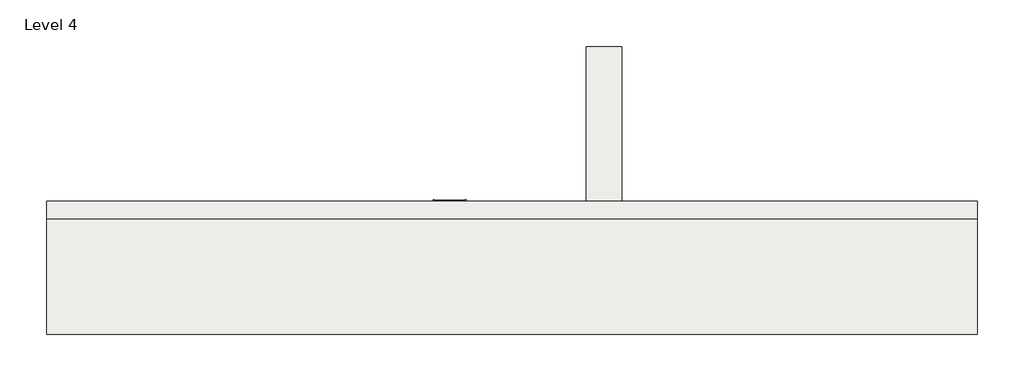
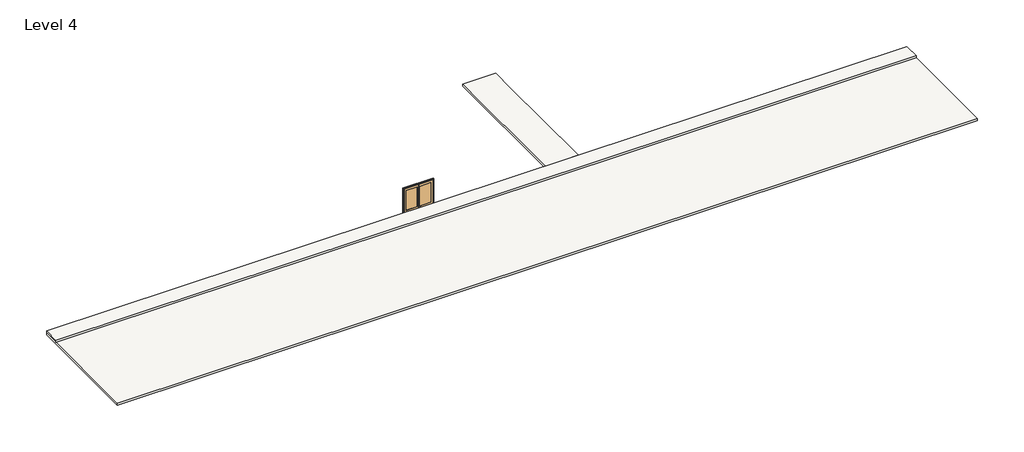
# One storey: 3 slabs, 1 door.
"""IFC4 building model written with IfcOpenShell, lengths in millimetres."""

from ifc_helpers import new_model, si_unit, frame, origin, place, context, project, spatial, polyline, outline, extrude, faceted_brep, transform, mapped, element, save
from components import garage_timber_side_hung_1_2271_x_2052mm_efc604d9

model = new_model("IFC4")

# Units and contexts
model_context = context("Model", 3, world=origin())
ifc_project = project(units=[si_unit("LENGTHUNIT", "METRE", prefix="MILLI")], contexts=[model_context])

# Site, building, storey
site = spatial("IfcSite", under=ifc_project)
building = spatial("IfcBuilding", under=site)
storey = spatial("IfcBuildingStorey", under=building, Name="Level 4", Elevation=-609.6)

# Door
placement = place(None, origin())
garage_timber_side_hung_1_2271_x_2052mm_shape = garage_timber_side_hung_1_2271_x_2052mm_efc604d9(model_context)
element("IfcDoor", 1, ObjectType="Garage - Timber Side Hung (1) : 2271 x 2052mm", at=placement, inside=storey, context=model_context, shape_type="MappedRepresentation", body=[
    mapped(garage_timber_side_hung_1_2271_x_2052mm_shape, transform((-4812.7201068, -6927.4122986, -609.6), x_axis=(-1.0, 0.0, 0.0), y_axis=(0.0, -1.0, 0.0), z_axis=(0.0, 0.0, 1.0))),
])

# Slabs
element("IfcSlab", 2, ObjectType="2' 3", at=placement, inside=storey, context=model_context, shape_type="SweptSolid", body=[
    extrude(outline(polyline([(31509.2798932, -7054.4122986), (31509.2798932, -16198.4122986), (-32536.8201068, -16198.4122986), (-32536.8201068, -7054.4122986), (31509.2798932, -7054.4122986)])), frame((0.0, 0.0, -762.0), z_axis=(0.0, 0.0, 1.0), x_axis=(1.0, 0.0, 0.0)), (0.0, 0.0, 1.0), 152.4),
])
element("IfcSlab", 3, ObjectType="2' 4", at=placement, inside=storey, context=model_context, shape_type="SweptSolid", body=[
    extrude(outline(polyline([(31509.2798932, -7054.4122986), (31509.2798932, -8273.6122986), (-32536.8201068, -8273.6122986), (-32536.8201068, -7054.4122986), (31509.2798932, -7054.4122986)])), frame((0.0, 0.0, -609.6), z_axis=(0.0, 0.0, 1.0), x_axis=(1.0, 0.0, 0.0)), (0.0, 0.0, 1.0), 152.4),
])
element("IfcSlab", 4, ObjectType="6\"", at=placement, inside=storey, context=model_context, shape_type="Brep", body=[
    faceted_brep([(7049.0798932, 3588.1877014, -609.6), (7049.0798932, -7054.4122986, -609.6), (4597.9798932, -7054.4122986, -609.6), (4597.9798932, 3588.1877014, -609.6), (7049.0798932, 3588.1877014, -457.2), (4597.9798932, 3588.1877014, -457.2), (4597.9798932, -7054.4122986, -457.2), (7049.0798932, -7054.4122986, -457.2), (7049.0798932, -6800.4122986, -457.2), (7049.0798932, 1746.6877014, -457.2)], [[[0, 1, 2, 3]], [[4, 5, 6, 7, 8, 9]], [[1, 0, 4, 9, 8, 7]], [[2, 1, 7, 6]], [[3, 2, 6, 5]], [[0, 3, 5, 4]]]),
])

save(model, "model.ifc")

# Revit data of these elements
# Type "Garage - Timber Side Hung (1) : 2271 x 2052mm"
#   Type Mark = "13"
#   Type Comments = "External Garage"
#   Operation = "DoubleDoorSingleSwing"
#   Manufacturer = "Revit"
#   Keynote = "L20"
#   Wrap Layers (Ext) from Ext = 0' - 4.03543"
#   Wrap Layers (Int) from Ext = 0' - 6.98819"
#   Thickness = 0' - 1.25984"
#   Stile Top Rail = 0' - 7.87402"
#   Stile Shutting = 0' - 3.93701"
#   Stile Lock Rail = 0' - 7.87402"
#   Stile Hanging = 0' - 6.88976"
#   Stile Bottom Rail = 0' - 9.84252"
#   Rough Width = 7' - 5.40945"
#   Rough Height = 6' - 8.7874"
#   O/A Frame Width = 0' - 2.51969"
#   Handle Z Distance = 3' - 5.33858"
#   Glazing Panel Height = 1' - 5.71654"
#   FrameWidth = 0' - 1.65354"
#   FrameOffset - External = 0' - 0.98425"
#   FrameDepth = 0' - 3.50394"
#   Door Panel Thickness = 0' - 1.25984"
#   Height = 6' - 8.7874"
#   Structural Tolerance = 0' - 0.31496"
#   Tolerance = 0' - 0.11811"
#   Undercut = 0' - 0.3937"
#   Width = 7' - 5.40945"
#   Cavity Closer Width = 0' - 1.9685"
#   Cavity Closer Offset from Ext = 0' - 4.03543"
#   Cavity Closer Depth = 0' - 2.95276"
#   Vis - Cavity Closers = yes
#   Function = 1
#   Material Door = Door - Panel
#   Wall Closure = (empty or 0)
# Type "2' 3"
#   Assembly Code = "B1010"
#   Function = 0
#   Layers, outside or top first: 0' - 6" "road" (function 1)
# Type "2' 4"
#   Assembly Code = "B1010"
#   Function = 0
#   Layers, outside or top first: 0' - 6" "road(1)" (function 1)
# Type "6\""
#   Assembly Code = "B1010"
#   Function = 0
#   Layers, outside or top first: 0' - 6" "0 floor outer" (function 1)
# Element 1 (IfcDoor, "Garage - Timber Side Hung (1) : 2271 x 2052mm")
#   Phase Created = New Construction
#   Materials on its faces: "Door - Panel"
# Element 2 (IfcSlab, "2' 3")
#   Height Offset From Level = 0' - 0"
#   Phase Created = New Construction
#   Materials on its faces: "road"
# Element 3 (IfcSlab, "2' 4")
#   Height Offset From Level = 0' - 6"
#   Phase Created = New Construction
#   Materials on its faces: "road(1)"
# Element 4 (IfcSlab, "6\"")
#   Height Offset From Level = 0' - 6"
#   Phase Created = New Construction
#   Materials on its faces: "0 floor outer", "0 olive green light"
# Materials
#   "Door - Panel": class "Wood", colour RGB 210 159 95, transparency 0, Cost = 0
#   "road": class "Generic", colour RGB 120 120 120, transparency 0, Cost = 0
#   "road(1)": class "Generic", colour RGB 120 120 120, transparency 0, Cost = 0
#   "0 floor outer": class "Generic", colour RGB 120 120 120, transparency 0, Cost = 0
#   "0 olive green light": class "Generic", colour RGB 120 120 120, transparency 0, Cost = 0
